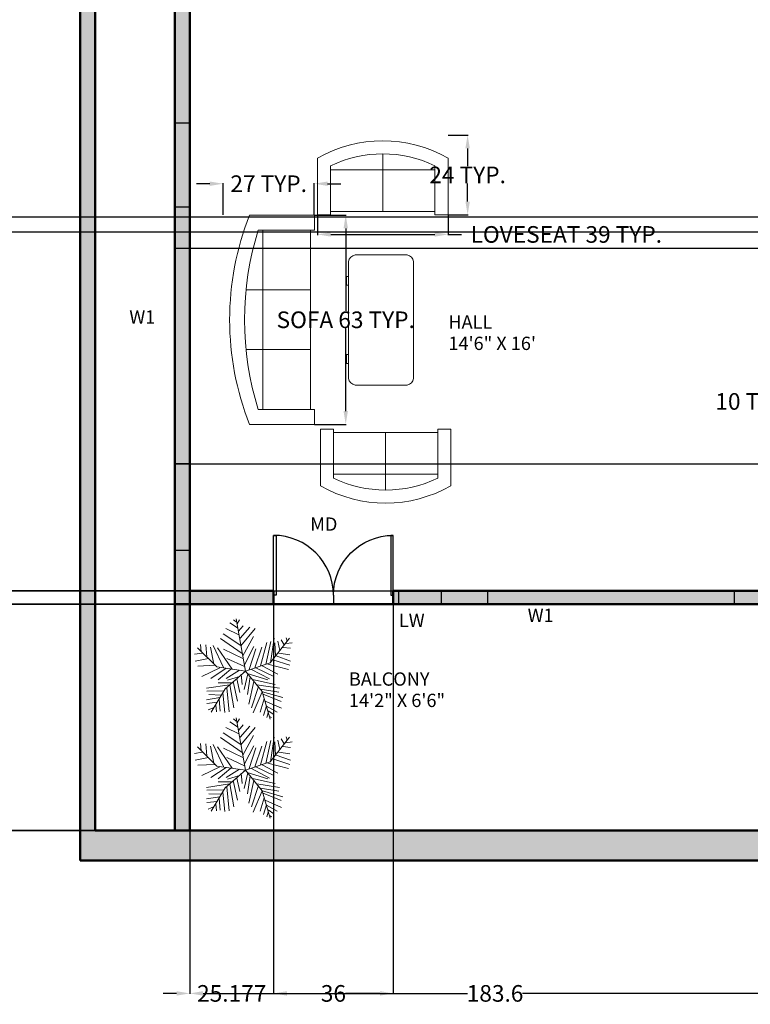
# Model space of a CAD drawing. Units: inches. Extents: x -12 to 887, y 330 to 874.
# Tile 5 of 9: x 442 to 662, y 330 to 626. Entities that reach past the tile are written whole.
import ezdxf

# ---------------------------------------------------------------- set-up
doc = ezdxf.new("R2010")
doc.units = ezdxf.units.IN
doc.header["$MEASUREMENT"] = 0
for name, color, linetype, lineweight in [('A-ANNO-DIMS', 2, 'Continuous', 18), ('A-ANNO-TEXT', 3, 'Continuous', 18), ('A-AREA-IDEN', 7, 'Continuous', 18), ('A-DOOR', 4, 'Continuous', 25), ('A-FURN', 9, 'Continuous', 18), ('A-GLAZ', 4, 'Continuous', 25), ('A-WALL', 7, 'Continuous', 50), ('A-WALL-PATT', 5, 'Continuous', 13), ('L-PLNT', 3, 'Continuous', 13)]:
    doc.layers.add(name, color=color, linetype=linetype, lineweight=lineweight)
doc.styles.get("Standard").update_dxf_attribs({"font": 'arial.ttf'})
doc.dimstyles.get("Standard").update_dxf_attribs({"dimtxt": 5, "dimasz": 4, "dimexe": 0.18, "dimexo": 0.0625, "dimgap": 0.09, "dimtad": 0, "dimtih": 1, "dimtoh": 1, "dimdec": 1, "dimzin": 0, "dimdsep": 46, "dimlunit": 4, "dimtxsty": 'Standard', "dimcen": 0.09, "dimadec": 0, "dimazin": 0, "dimtfac": 1, "dimtdec": 1, "dimtofl": 0, "dimtmove": 0, "dimatfit": 3, "dimfxl": 1, "dimtolj": 1, "dimtzin": 0, "dimarcsym": 0})

# ---------------------------------------------------------------- blocks, each defined once
blk = doc.blocks.new('*U5')
for p, q in [((0, 0), (0, -6)), ((40, 0), (40, -6))]:
    blk.add_line(p, q)
blk.add_lwpolyline([(0, 0), (0, 40), (1.75, 40), (1.75, 0)], close=True)
blk.add_arc((0, 0), 40, 0, 90)
blk = doc.blocks.new('Sofa - Roundback 7 ft.')
for p, q in [((-12.00002, -32.4421), (-12.00003, -6.5971)), ((11.99997, -32.4421), (11.99998, -6.5971)), ((-36.000027, -34), (-36.000027, -11.4696)), ((35.99998, -34), (35.99998, -11.4696)), ((-35.999844, -13.3819), (35.9998, -13.3819)), ((-36.000027, -32.4421), (35.99998, -32.4421))]:
    blk.add_line(p, q)
for points in [[(-36.000027, -34), (-42.000027, -34), (-42.000027, -8)], [(41.99998, -8), (41.99998, -34), (35.99998, -34)]]:
    blk.add_lwpolyline(points)
for centre, radius, start, end in [((0, -114.25), 114.25, 68.43141, 111.5686), ((-0.00001, -127.1968), 121.1968, 72.72033, 107.2797)]:
    blk.add_arc(centre, radius, start, end)
blk = doc.blocks.new('Sofa - Roundback Loveseat 5 ft.')
for p, q in [((0, -32.44198), (0, -5.99998)), ((-24, -33.99998), (-24, -11.46958)), ((-23.9998, -13.38178), (23.99986, -13.38178)), ((24.00004, -33.99998), (24.00004, -11.46958)), ((-24, -32.44198), (24.00004, -32.44198))]:
    blk.add_line(p, q)
for points in [[(-24, -33.99998), (-30, -33.99998), (-30, -7.99998)], [(30.00004, -7.99998), (30.00004, -33.99998), (24.00004, -33.99998)]]:
    blk.add_lwpolyline(points)
for centre, radius, start, end in [((0, -60.24998), 60.24998, 60.13715, 119.8628), ((0, -61.38438), 55.38444, 64.32083, 115.6792)]:
    blk.add_arc(centre, radius, start, end)
blk = doc.blocks.new('Desk - 30 x 60 in.')
for p, q in [((-26.999995, 0), (26.999995, 0)), ((-29.999995, -27), (-29.999995, -3)), ((29.999995, -3), (29.999995, -27)), ((26.999995, -30), (-26.999995, -30)), ((-20.000005, -30), (-20.000005, -31)), ((-20.000005, -31), (-16.000005, -31)), ((-16.000005, -31), (-16.000005, -30)), ((15.999995, -31), (15.999995, -30)), ((19.999995, -31), (15.999995, -31)), ((19.999995, -30), (19.999995, -31))]:
    blk.add_line(p, q)
for centre, start, end in [((-26.499995, -3.5), 98.1301, 171.8699), ((26.499995, -3.5), 8.130102, 81.8699), ((-26.499995, -26.5), 188.1301, 261.8699), ((26.499995, -26.5), 278.1301, 351.8699)]:
    blk.add_arc(centre, 3.535534, start, end)
blk = doc.blocks.new('*U14')
for p, q in [((-258.7244, 1362.456), (-332.3336, 1421.4348)), ((0, 0), (-266.7, 1447.8)), ((-231.1146, 1315.2628), (-166.7002, 1421.4348)), ((-185.1152, 1008.5578), (-553.1612, 1185.4942)), ((-221.9198, 1197.3052), (-433.5526, 1338.8594)), ((-194.31, 1102.9442), (-65.4812, 1256.284)), ((-148.3106, 914.1968), (118.5418, 1220.9018)), ((-129.8956, 701.8528), (265.7602, 1185.4942)), ((-93.091, 489.5342), (-700.3796, 902.3858)), ((-129.8956, 713.6638), (-626.7704, 1032.1544)), ((-74.7014, 418.7444), (219.7608, 961.39)), ((560.197, 182.8292), (698.2206, 819.8358)), ((685.8, 228.6), (1219.2, 914.4)), ((689.0258, 230.0224), (790.2448, 914.1968)), ((891.4384, 831.6214), (946.658, 572.1096)), ((983.4626, 867.0036), (1066.2666, 725.4494)), ((1121.4862, 925.9824), (1149.0706, 831.6214)), ((-800.1, 114.3), (-1333.5, 647.7)), ((-1234.059, 536.7274), (-1252.4486, 737.2604)), ((-1105.2302, 725.4494), (-1077.6458, 395.1732)), ((-976.4268, 666.4706), (-884.4026, 194.6402)), ((-902.8176, 713.6638), (-617.5756, 100.2538)), ((-369.1382, 53.086), (-783.1836, 642.874)), ((-617.5756, 607.4918), (-74.7014, 347.98)), ((-28.6766, 171.0436), (228.9556, 678.2816)), ((100.1268, 41.275), (284.1498, 619.2774)), ((256.5654, 88.4682), (449.7832, 666.4706)), ((412.9786, 147.447), (587.8068, 796.2392)), ((808.6344, 784.4282), (827.0494, 418.7444)), ((1029.462, 654.685), (1241.0948, 631.0884)), ((1112.2914, 760.8316), (1296.3144, 784.4282)), ((-1206.4492, 501.3198), (-1418.082, 465.9376)), ((-1031.621, 347.98), (-1399.667, 277.1902)), ((-525.5514, 347.98), (-28.6766, 123.8504)), ((753.4148, 312.5978), (1222.6798, 159.2326)), ((845.439, 418.7444), (1241.0948, 277.1902)), ((919.0482, 501.3198), (1222.6798, 454.152)), ((-847.598, 159.2326), (-1326.0578, 135.636)), ((-718.7946, 88.4682), (-1215.644, -147.447)), ((-543.9664, 76.6572), (-967.2066, -206.4512)), ((0, 0), (-800.1, 114.3)), ((-405.9428, 53.086), (-764.794, -241.8334)), ((0, 0), (-571.5, -495.3)), ((-166.7002, 29.4894), (-543.9664, -206.4512)), ((0, 0), (685.8, 228.6)), ((0, 0), (457.2, -571.5)), ((164.5412, 41.275), (661.416, -218.2368)), ((284.1498, 88.4682), (781.0246, -147.447)), ((458.978, 147.447), (891.4384, -88.4682)), ((615.4166, 194.6402), (1185.8752, 41.275)), ((-166.7002, -147.447), (-507.1618, -253.619)), ((-240.3094, -218.2368), (-157.5054, -595.7062)), ((-120.7008, -88.4682), (-93.091, -371.5766)), ((63.3222, -76.6826), (-37.8714, -513.1308)), ((44.9326, -64.897), (615.4166, -241.8334)), ((127.7366, -159.258), (54.1274, -654.685)), ((192.151, -230.0224), (817.8292, -371.5766)), ((-442.7474, -383.3876), (-1086.8406, -477.7486)), ((-571.5, -495.3), (-952.5, -1143)), ((-387.5278, -324.4088), (-764.794, -324.4088)), ((-525.5514, -465.963), (-451.9422, -1126.5408)), ((-433.5526, -383.3876), (-323.1134, -1020.3688)), ((-341.5284, -289.0012), (-221.9198, -831.6214)), ((228.9556, -289.0012), (90.932, -914.1968)), ((357.759, -430.5554), (164.5412, -1020.3688)), ((311.7596, -383.3876), (937.4378, -477.7486)), ((412.9786, -501.3452), (919.0482, -583.9206)), ((-718.7946, -737.2604), (-1086.8406, -796.2392)), ((-617.5756, -548.5384), (-1077.6458, -560.324)), ((-681.9646, -666.496), (-1022.4262, -654.685)), ((-737.1842, -784.4536), (-709.5744, -1114.7298)), ((-635.9652, -607.5172), (-580.771, -1150.1374)), ((458.978, -572.1096), (210.5406, -1161.923)), ((514.1976, -772.6426), (403.7838, -1138.3264)), ((457.2, -571.5), (685.8, -1333.5)), ((468.1982, -572.1096), (1029.462, -737.2604)), ((486.5878, -642.8994), (983.4626, -843.4324)), ((-783.1836, -867.029), (-1077.6458, -902.4112)), ((-875.2078, -1008.5832), (-1040.8412, -1079.3476)), ((-829.2084, -937.7934), (-810.7934, -1126.5408)), ((578.612, -961.39), (495.7826, -1232.7128)), ((541.8074, -831.6214), (992.6574, -1032.1544)), ((578.612, -973.1756), (873.0488, -1138.3264)), ((624.6114, -1161.923), (587.8068, -1291.6916)), ((624.6114, -1102.9442), (781.0246, -1209.1162)), ((679.8056, -1268.095), (716.6102, -1291.6916))]:
    blk.add_line(p, q)
blk = doc.blocks.new('*D19')
at = {"layer": 'A-ANNO-DIMS', "color": 0, "lineweight": -2, "transparency": 16777216}
for p, q in [((678.65, 512.63), (678.65, 510.96)), ((688.99, 512.63), (688.99, 510.96)), ((678.65, 511.14), (674.65, 511.14)), ((684.99, 511.14), (682.65, 511.14))]:
    blk.add_line(p, q, dxfattribs=at)
at = {"layer": 'A-ANNO-DIMS', "color": 0, "transparency": 16777216}
for points in [[(682.65, 511.8), (682.65, 510.47), (678.65, 511.14)], [(684.99, 511.8), (684.99, 510.47), (688.99, 511.14)]]:
    blk.add_solid(points, dxfattribs=at)
at = {"layer": 'Defpoints', "color": 0, "transparency": 16777216}
for p in [(678.65, 512.69), (688.99, 512.69), (678.65, 511.14)]:
    blk.add_point(p, dxfattribs=at)
at = {"layer": 'A-ANNO-DIMS', "color": 0, "transparency": 16777216, "insert": (662.62, 511.14), "char_height": 5, "attachment_point": 5}
blk.add_mtext('\\A1;10 TYP.', dxfattribs=at)
blk = doc.blocks.new('*D30')
at = {"layer": 'A-ANNO-DIMS', "color": 0, "lineweight": -2, "transparency": 16777216}
for p, q in [((530.58, 567.16), (540.13, 567.16)), ((539.95, 563.16), (539.95, 538.37)), ((539.95, 508.23), (539.95, 533.02)), ((530.58, 504.23), (540.13, 504.23))]:
    blk.add_line(p, q, dxfattribs=at)
at = {"layer": 'A-ANNO-DIMS', "color": 0, "transparency": 16777216}
for points in [[(539.29, 563.16), (540.62, 563.16), (539.95, 567.16)], [(539.29, 508.23), (540.62, 508.23), (539.95, 504.23)]]:
    blk.add_solid(points, dxfattribs=at)
at = {"layer": 'Defpoints', "color": 0, "transparency": 16777216}
for p in [(530.51, 567.16), (539.95, 567.16), (530.51, 504.23)]:
    blk.add_point(p, dxfattribs=at)
at = {"layer": 'A-ANNO-DIMS', "color": 0, "transparency": 16777216, "insert": (539.95, 535.69), "char_height": 5, "attachment_point": 5}
blk.add_mtext('\\A1;SOFA 63 TYP.', dxfattribs=at)
blk = doc.blocks.new('*D31')
at = {"layer": 'A-ANNO-DIMS', "color": 0, "lineweight": -2, "transparency": 16777216}
for p, q in [((499.05, 576.6), (495.05, 576.6)), ((503.05, 567.22), (503.05, 576.78)), ((530.51, 567.22), (530.51, 576.78)), ((534.51, 576.6), (538.51, 576.6))]:
    blk.add_line(p, q, dxfattribs=at)
at = {"layer": 'A-ANNO-DIMS', "color": 0, "transparency": 16777216}
for points in [[(499.05, 577.26), (499.05, 575.93), (503.05, 576.6)], [(534.51, 577.26), (534.51, 575.93), (530.51, 576.6)]]:
    blk.add_solid(points, dxfattribs=at)
at = {"layer": 'Defpoints', "color": 0, "transparency": 16777216}
for p in [(503.05, 576.6), (503.05, 567.16), (530.51, 567.16)]:
    blk.add_point(p, dxfattribs=at)
at = {"layer": 'A-ANNO-DIMS', "color": 0, "transparency": 16777216, "insert": (516.78, 576.6), "char_height": 5, "attachment_point": 5}
blk.add_mtext('\\A1;27 TYP.', dxfattribs=at)
blk = doc.blocks.new('*D32')
at = {"layer": 'A-ANNO-DIMS', "color": 0, "lineweight": -2, "transparency": 16777216}
for p, q in [((531.45, 567.18), (531.45, 561.17)), ((570.72, 567.18), (570.72, 561.17)), ((535.45, 561.35), (566.72, 561.35)), ((570.72, 561.35), (574.72, 561.35))]:
    blk.add_line(p, q, dxfattribs=at)
at = {"layer": 'A-ANNO-DIMS', "color": 0, "transparency": 16777216}
for points in [[(535.45, 562.02), (535.45, 560.68), (531.45, 561.35)], [(566.72, 562.02), (566.72, 560.68), (570.72, 561.35)]]:
    blk.add_solid(points, dxfattribs=at)
at = {"layer": 'Defpoints', "color": 0, "transparency": 16777216}
for p in [(531.45, 567.24), (570.72, 567.24), (570.72, 561.35)]:
    blk.add_point(p, dxfattribs=at)
at = {"layer": 'A-ANNO-DIMS', "color": 0, "transparency": 16777216, "insert": (606.28, 561.35), "char_height": 5, "attachment_point": 5}
blk.add_mtext('\\A1;LOVESEAT 39 TYP.', dxfattribs=at)
blk = doc.blocks.new('*D33')
at = {"layer": 'A-ANNO-DIMS', "color": 0, "lineweight": -2, "transparency": 16777216}
for p, q in [((570.78, 591.23), (576.79, 591.23)), ((576.61, 587.23), (576.61, 581.84)), ((576.61, 571.24), (576.61, 576.63)), ((570.78, 567.24), (576.79, 567.24))]:
    blk.add_line(p, q, dxfattribs=at)
at = {"layer": 'A-ANNO-DIMS', "color": 0, "transparency": 16777216}
for points in [[(575.94, 587.23), (577.28, 587.23), (576.61, 591.23)], [(575.94, 571.24), (577.28, 571.24), (576.61, 567.24)]]:
    blk.add_solid(points, dxfattribs=at)
at = {"layer": 'Defpoints', "color": 0, "transparency": 16777216}
for p in [(570.72, 591.23), (576.61, 591.23), (570.72, 567.24)]:
    blk.add_point(p, dxfattribs=at)
at = {"layer": 'A-ANNO-DIMS', "color": 0, "transparency": 16777216, "insert": (576.61, 579.24), "char_height": 5, "attachment_point": 5}
blk.add_mtext('\\A1;24 TYP.', dxfattribs=at)
blk = doc.blocks.new('*D60')
at = {"layer": 'A-ANNO-DIMS', "color": 0, "lineweight": -2, "transparency": 16777216}
for p, q in [((383.99, 450.16), (873.75, 450.16)), ((873.57, 446.16), (873.57, 418.8)), ((873.57, 386.16), (873.57, 413.52)), ((383.99, 382.16), (873.75, 382.16))]:
    blk.add_line(p, q, dxfattribs=at)
at = {"layer": 'A-ANNO-DIMS', "color": 0, "transparency": 16777216}
for points in [[(872.9, 446.16), (874.24, 446.16), (873.57, 450.16)], [(872.9, 386.16), (874.24, 386.16), (873.57, 382.16)]]:
    blk.add_solid(points, dxfattribs=at)
at = {"layer": 'Defpoints', "color": 0, "transparency": 16777216}
for p in [(383.93, 450.16), (873.57, 450.16), (383.93, 382.16)]:
    blk.add_point(p, dxfattribs=at)
at = {"layer": 'A-ANNO-DIMS', "color": 0, "transparency": 16777216, "insert": (873.57, 416.16), "char_height": 5, "attachment_point": 5}
blk.add_mtext('\\A1;68', dxfattribs=at)
blk = doc.blocks.new('*D61')
at = {"layer": 'A-ANNO-DIMS', "color": 0, "lineweight": -2, "transparency": 16777216}
for p, q in [((873.57, 458.16), (873.57, 462.16)), ((873.57, 462.16), (877.57, 462.16)), ((383.99, 454.16), (873.75, 454.16)), ((383.99, 450.16), (873.75, 450.16)), ((873.57, 446.16), (873.57, 442.16))]:
    blk.add_line(p, q, dxfattribs=at)
at = {"layer": 'A-ANNO-DIMS', "color": 0, "transparency": 16777216}
for points in [[(872.9, 458.16), (874.24, 458.16), (873.57, 454.16)], [(872.9, 446.16), (874.24, 446.16), (873.57, 450.16)]]:
    blk.add_solid(points, dxfattribs=at)
at = {"layer": 'Defpoints', "color": 0, "transparency": 16777216}
for p in [(383.93, 454.16), (873.57, 454.16), (383.93, 450.16)]:
    blk.add_point(p, dxfattribs=at)
at = {"layer": 'A-ANNO-DIMS', "color": 0, "transparency": 16777216, "insert": (879.39, 462.16), "char_height": 5, "attachment_point": 5}
blk.add_mtext('\\A1;4', dxfattribs=at)
blk = doc.blocks.new('*D62')
at = {"layer": 'A-ANNO-DIMS', "color": 0, "lineweight": -2, "transparency": 16777216}
for p, q in [((383.99, 562.16), (873.75, 562.16)), ((873.57, 558.16), (873.57, 510.8)), ((873.57, 458.16), (873.57, 505.52)), ((383.99, 454.16), (873.75, 454.16))]:
    blk.add_line(p, q, dxfattribs=at)
at = {"layer": 'A-ANNO-DIMS', "color": 0, "transparency": 16777216}
for points in [[(872.9, 558.16), (874.24, 558.16), (873.57, 562.16)], [(872.9, 458.16), (874.24, 458.16), (873.57, 454.16)]]:
    blk.add_solid(points, dxfattribs=at)
at = {"layer": 'Defpoints', "color": 0, "transparency": 16777216}
for p in [(383.93, 562.16), (873.57, 562.16), (383.93, 454.16)]:
    blk.add_point(p, dxfattribs=at)
at = {"layer": 'A-ANNO-DIMS', "color": 0, "transparency": 16777216, "insert": (873.57, 508.16), "char_height": 5, "attachment_point": 5}
blk.add_mtext('\\A1;108', dxfattribs=at)
blk = doc.blocks.new('*D63')
at = {"layer": 'A-ANNO-DIMS', "color": 0, "lineweight": -2, "transparency": 16777216}
for p, q in [((873.57, 570.66), (873.57, 574.66)), ((873.57, 574.66), (877.57, 574.66)), ((383.99, 566.66), (873.75, 566.66)), ((383.99, 562.16), (873.75, 562.16)), ((873.57, 558.16), (873.57, 554.16))]:
    blk.add_line(p, q, dxfattribs=at)
at = {"layer": 'A-ANNO-DIMS', "color": 0, "transparency": 16777216}
for points in [[(872.9, 570.66), (874.24, 570.66), (873.57, 566.66)], [(872.9, 558.16), (874.24, 558.16), (873.57, 562.16)]]:
    blk.add_solid(points, dxfattribs=at)
at = {"layer": 'Defpoints', "color": 0, "transparency": 16777216}
for p in [(383.93, 566.66), (873.57, 566.66), (383.93, 562.16)]:
    blk.add_point(p, dxfattribs=at)
at = {"layer": 'A-ANNO-DIMS', "color": 0, "transparency": 16777216, "insert": (882.33, 574.66), "char_height": 5, "attachment_point": 5}
blk.add_mtext('\\A1;4.5', dxfattribs=at)
blk = doc.blocks.new('*D64')
at = {"layer": 'A-ANNO-DIMS', "color": 0, "lineweight": -2, "transparency": 16777216}
for p, q in [((383.99, 685.16), (873.75, 685.16)), ((873.57, 681.16), (873.57, 628.55)), ((873.57, 570.66), (873.57, 623.27)), ((383.99, 566.66), (873.75, 566.66))]:
    blk.add_line(p, q, dxfattribs=at)
at = {"layer": 'A-ANNO-DIMS', "color": 0, "transparency": 16777216}
for points in [[(872.9, 681.16), (874.24, 681.16), (873.57, 685.16)], [(872.9, 570.66), (874.24, 570.66), (873.57, 566.66)]]:
    blk.add_solid(points, dxfattribs=at)
at = {"layer": 'Defpoints', "color": 0, "transparency": 16777216}
for p in [(383.93, 685.16), (873.57, 685.16), (383.93, 566.66)]:
    blk.add_point(p, dxfattribs=at)
at = {"layer": 'A-ANNO-DIMS', "color": 0, "transparency": 16777216, "insert": (873.57, 625.91), "char_height": 5, "attachment_point": 5}
blk.add_mtext('\\A1;118.5', dxfattribs=at)
blk = doc.blocks.new('*D95')
at = {"layer": 'A-ANNO-DIMS', "color": 0, "lineweight": -2, "transparency": 16777216}
for p, q in [((493.07, 382.1), (493.07, 332.98)), ((676.66, 382.1), (676.66, 332.98)), ((497.07, 333.16), (576.57, 333.16)), ((672.66, 333.16), (593.15, 333.16))]:
    blk.add_line(p, q, dxfattribs=at)
at = {"layer": 'A-ANNO-DIMS', "color": 0, "transparency": 16777216}
for points in [[(497.07, 333.83), (497.07, 332.49), (493.07, 333.16)], [(672.66, 333.83), (672.66, 332.49), (676.66, 333.16)]]:
    blk.add_solid(points, dxfattribs=at)
at = {"layer": 'Defpoints', "color": 0, "transparency": 16777216}
for p in [(493.07, 382.16), (676.66, 382.16), (676.66, 333.16)]:
    blk.add_point(p, dxfattribs=at)
at = {"layer": 'A-ANNO-DIMS', "color": 0, "transparency": 16777216, "insert": (584.86, 333.16), "char_height": 5, "attachment_point": 5}
blk.add_mtext('\\A1;183.6', dxfattribs=at)
blk = doc.blocks.new('*D98')
at = {"layer": 'A-ANNO-DIMS', "color": 0, "lineweight": -2, "transparency": 16777216}
for p, q in [((460.13, 830.66), (873.75, 830.66)), ((873.57, 826.66), (873.57, 604.54)), ((873.57, 377.16), (873.57, 599.28)), ((460.13, 373.16), (873.75, 373.16))]:
    blk.add_line(p, q, dxfattribs=at)
at = {"layer": 'A-ANNO-DIMS', "color": 0, "transparency": 16777216}
for points in [[(872.9, 826.66), (874.24, 826.66), (873.57, 830.66)], [(872.9, 377.16), (874.24, 377.16), (873.57, 373.16)]]:
    blk.add_solid(points, dxfattribs=at)
at = {"layer": 'Defpoints', "color": 0, "transparency": 16777216}
for p in [(460.07, 830.66), (873.57, 830.66), (460.07, 373.16)]:
    blk.add_point(p, dxfattribs=at)
at = {"layer": 'A-ANNO-DIMS', "color": 0, "transparency": 16777216, "insert": (873.57, 601.91), "char_height": 5, "attachment_point": 5}
blk.add_mtext('\\A1;457.5', dxfattribs=at)
blk = doc.blocks.new('*D99')
at = {"layer": 'A-ANNO-DIMS', "color": 0, "lineweight": -2, "transparency": 16777216}
for p, q in [((493.01, 450.16), (1.75, 450.16)), ((1.93, 446.16), (1.93, 418.8)), ((1.93, 386.16), (1.93, 413.52)), ((493.01, 382.16), (1.75, 382.16))]:
    blk.add_line(p, q, dxfattribs=at)
at = {"layer": 'A-ANNO-DIMS', "color": 0, "transparency": 16777216}
for points in [[(1.26, 446.16), (2.59, 446.16), (1.93, 450.16)], [(1.26, 386.16), (2.59, 386.16), (1.93, 382.16)]]:
    blk.add_solid(points, dxfattribs=at)
at = {"layer": 'Defpoints', "color": 0, "transparency": 16777216}
for p in [(1.93, 450.16), (493.07, 450.16), (493.07, 382.16)]:
    blk.add_point(p, dxfattribs=at)
at = {"layer": 'A-ANNO-DIMS', "color": 0, "transparency": 16777216, "insert": (1.93, 416.16), "char_height": 5, "attachment_point": 5}
blk.add_mtext('\\A1;68', dxfattribs=at)
blk = doc.blocks.new('*D100')
at = {"layer": 'A-ANNO-DIMS', "color": 0, "lineweight": -2, "transparency": 16777216}
for p, q in [((1.93, 458.16), (1.93, 462.16)), ((1.93, 462.16), (5.93, 462.16)), ((493.01, 454.16), (1.75, 454.16)), ((493.01, 450.16), (1.75, 450.16)), ((1.93, 446.16), (1.93, 442.16))]:
    blk.add_line(p, q, dxfattribs=at)
at = {"layer": 'A-ANNO-DIMS', "color": 0, "transparency": 16777216}
for points in [[(1.26, 458.16), (2.59, 458.16), (1.93, 454.16)], [(1.26, 446.16), (2.59, 446.16), (1.93, 450.16)]]:
    blk.add_solid(points, dxfattribs=at)
at = {"layer": 'Defpoints', "color": 0, "transparency": 16777216}
for p in [(1.93, 454.16), (493.07, 454.16), (493.07, 450.16)]:
    blk.add_point(p, dxfattribs=at)
at = {"layer": 'A-ANNO-DIMS', "color": 0, "transparency": 16777216, "insert": (7.75, 462.16), "char_height": 5, "attachment_point": 5}
blk.add_mtext('\\A1;4', dxfattribs=at)
blk = doc.blocks.new('*D101')
at = {"layer": 'A-ANNO-DIMS', "color": 0, "lineweight": -2, "transparency": 16777216}
for p, q in [((493.01, 643.16), (1.75, 643.16)), ((1.93, 639.16), (1.93, 551.3)), ((1.93, 458.16), (1.93, 546.02)), ((493.01, 454.16), (1.75, 454.16))]:
    blk.add_line(p, q, dxfattribs=at)
at = {"layer": 'A-ANNO-DIMS', "color": 0, "transparency": 16777216}
for points in [[(1.26, 639.16), (2.59, 639.16), (1.93, 643.16)], [(1.26, 458.16), (2.59, 458.16), (1.93, 454.16)]]:
    blk.add_solid(points, dxfattribs=at)
at = {"layer": 'Defpoints', "color": 0, "transparency": 16777216}
for p in [(1.93, 643.16), (493.07, 643.16), (493.07, 454.16)]:
    blk.add_point(p, dxfattribs=at)
at = {"layer": 'A-ANNO-DIMS', "color": 0, "transparency": 16777216, "insert": (1.93, 548.66), "char_height": 5, "attachment_point": 5}
blk.add_mtext('\\A1;189', dxfattribs=at)
blk = doc.blocks.new('*D120')
at = {"layer": 'A-ANNO-DIMS', "color": 0, "lineweight": -2, "transparency": 16777216}
for p, q in [((518.25, 454.1), (518.25, 332.98)), ((554.25, 454.1), (554.25, 332.98)), ((522.25, 333.16), (532.58, 333.16)), ((550.25, 333.16), (539.91, 333.16))]:
    blk.add_line(p, q, dxfattribs=at)
at = {"layer": 'A-ANNO-DIMS', "color": 0, "transparency": 16777216}
for points in [[(522.25, 333.83), (522.25, 332.49), (518.25, 333.16)], [(550.25, 333.83), (550.25, 332.49), (554.25, 333.16)]]:
    blk.add_solid(points, dxfattribs=at)
at = {"layer": 'Defpoints', "color": 0, "transparency": 16777216}
for p in [(518.25, 454.16), (554.25, 454.16), (554.25, 333.16)]:
    blk.add_point(p, dxfattribs=at)
at = {"layer": 'A-ANNO-DIMS', "color": 0, "transparency": 16777216, "insert": (536.25, 333.16), "char_height": 5, "attachment_point": 5}
blk.add_mtext('\\A1;36', dxfattribs=at)
blk = doc.blocks.new('*D121')
at = {"layer": 'A-ANNO-DIMS', "color": 0, "lineweight": -2, "transparency": 16777216}
for p, q in [((493.07, 454.1), (493.07, 332.98)), ((518.25, 454.1), (518.25, 332.98)), ((489.07, 333.16), (485.07, 333.16)), ((522.25, 333.16), (526.25, 333.16))]:
    blk.add_line(p, q, dxfattribs=at)
at = {"layer": 'A-ANNO-DIMS', "color": 0, "transparency": 16777216}
for points in [[(489.07, 333.83), (489.07, 332.49), (493.07, 333.16)], [(522.25, 333.83), (522.25, 332.49), (518.25, 333.16)]]:
    blk.add_solid(points, dxfattribs=at)
at = {"layer": 'Defpoints', "color": 0, "transparency": 16777216}
for p in [(493.07, 454.16), (518.25, 454.16), (518.25, 333.16)]:
    blk.add_point(p, dxfattribs=at)
at = {"layer": 'A-ANNO-DIMS', "color": 0, "transparency": 16777216, "insert": (505.66, 333.16), "char_height": 5, "attachment_point": 5}
blk.add_mtext('\\A1;25.177', dxfattribs=at)
blk = doc.blocks.new('*D129')
at = {"layer": 'A-ANNO-DIMS', "color": 0, "lineweight": -2, "transparency": 16777216}
for p, q in [((488.63, 557.26), (873.75, 557.26)), ((873.57, 553.26), (873.57, 527.44)), ((873.57, 496.34), (873.57, 522.16)), ((488.63, 492.34), (873.75, 492.34))]:
    blk.add_line(p, q, dxfattribs=at)
at = {"layer": 'A-ANNO-DIMS', "color": 0, "transparency": 16777216}
for points in [[(872.9, 553.26), (874.24, 553.26), (873.57, 557.26)], [(872.9, 496.34), (874.24, 496.34), (873.57, 492.34)]]:
    blk.add_solid(points, dxfattribs=at)
at = {"layer": 'Defpoints', "color": 0, "transparency": 16777216}
for p in [(488.57, 557.26), (488.57, 492.34), (873.57, 492.34)]:
    blk.add_point(p, dxfattribs=at)
at = {"layer": 'A-ANNO-DIMS', "color": 0, "transparency": 16777216, "insert": (873.57, 524.8), "char_height": 5, "attachment_point": 5}
blk.add_mtext('\\A1;64.91', dxfattribs=at)

msp = doc.modelspace()

# ---------------------------------------------------------------- hatches: boundary and pattern name
at = {"layer": 'A-WALL-PATT'}
h = msp.add_hatch(color=256, dxfattribs=at)
h.dxf.hatch_style = 1
h.paths.add_polyline_path([(94.575, 830.6611), (67.3199, 830.6611), (67.3199, 821.6611), (70.4263, 821.6611), (79.4263, 821.6611), (94.575, 821.6611)])
h.paths.add_polyline_path([(288.8031, 830.6611), (257.9263, 830.6611), (253.4263, 830.6611), (253.4263, 821.6611), (288.8031, 821.6611)])
h.paths.add_polyline_path([(74.9263, 696.9265), (70.4263, 696.9265), (70.4263, 678.4656), (74.9263, 678.4656)])
h.paths.add_polyline_path([(74.9263, 584.8756), (70.4263, 584.8756), (70.4263, 562.1611), (74.9263, 562.1611)])
h.paths.add_polyline_path([(135.5357, 566.6611), (122.6994, 566.6611), (122.6994, 562.1611), (135.5357, 562.1611)])
h.paths.add_polyline_path([(257.9263, 579.1607), (253.4263, 579.1607), (253.4263, 562.1611), (257.9263, 562.1611)])
h.paths.add_polyline_path([(272.0195, 454.1611), (254.2006, 454.1611), (254.2006, 450.1611), (272.0195, 450.1611)])
h.paths.add_polyline_path([(392.9263, 454.1611), (374.959, 454.1611), (374.959, 450.1611), (383.9263, 450.1611), (392.9263, 450.1611)])
h.paths.add_polyline_path([(493.0683, 466.4171), (488.5683, 466.4171), (488.5683, 450.1611), (493.0683, 450.1611)])
h.paths.add_polyline_path([(568.6302, 454.1611), (555.938, 454.1611), (555.938, 450.1611), (568.6302, 450.1611)])
h.paths.add_polyline_path([(493.0683, 594.9471), (488.5683, 594.9471), (488.5683, 569.5862), (493.0683, 569.5862)])
h.paths.add_polyline_path([(690.1615, 454.1611), (672.3426, 454.1611), (672.3426, 450.1611), (690.1615, 450.1611)])
h.paths.add_polyline_path([(811.0683, 454.1611), (793.101, 454.1611), (793.101, 450.1611), (802.0683, 450.1611), (811.0683, 450.1611)])
h.paths.add_polyline_path([(811.0683, 578.3606), (802.0683, 578.3606), (802.0683, 566.6611), (802.0683, 553.5254), (811.0683, 553.5254)])
h.paths.add_polyline_path([(811.0683, 701.6611), (802.0683, 701.6611), (802.0683, 689.9616), (802.0683, 676.8259), (811.0683, 676.8259)])
h.paths.add_polyline_path([(811.0683, 830.6611), (782.165, 830.6611), (782.165, 821.6611), (802.0683, 821.6611), (811.0683, 821.6611)])
h.paths.add_polyline_path([(706.9451, 830.6611), (671.5683, 830.6611), (671.5683, 821.6611), (706.9451, 821.6611)])
h.paths.add_polyline_path([(512.717, 830.6611), (485.4619, 830.6611), (485.4619, 821.6611), (488.5683, 821.6611), (512.717, 821.6611)])
h.paths.add_polyline_path([(392.9263, 697.8668), (383.9263, 697.8668), (383.9263, 689.6611), (383.9263, 676.5034), (392.9263, 676.5034)])
h.paths.add_polyline_path([(392.9263, 830.6611), (364.023, 830.6611), (364.023, 821.7357), (392.9263, 821.7357)])
h.paths.add_polyline_path([(392.9263, 619.0434), (383.9263, 619.0434), (383.9263, 588.7499), (392.9263, 588.7499)])
h.paths.add_polyline_path([(392.9263, 578.3606), (383.9263, 578.3606), (383.9263, 566.6611), (383.9263, 553.5254), (392.9263, 553.5254)])
h.paths.add_polyline_path([(257.9263, 699.8547), (253.4263, 699.8547), (253.4263, 697.1611), (253.4263, 677.338), (257.9263, 677.338)])
h.paths.add_polyline_path([(493.0683, 714.3785), (488.5683, 714.3785), (488.5683, 689.6611), (493.0683, 689.6611)])
h.paths.add_polyline_path([(74.9263, 491.4191), (70.4263, 491.4191), (70.4263, 480.7097), (74.9263, 480.7097)])
h = msp.add_hatch(color=256, dxfattribs=at)
h.dxf.hatch_style = 1
h.paths.add_polyline_path([(671.5683, 830.6611), (512.717, 830.6611), (512.717, 821.6611), (617.0825, 821.6611), (617.0825, 797.5825), (617.0787, 783.3094), (621.5683, 783.3094), (621.5683, 821.6611), (671.5683, 821.6611)], flags=17)
h.paths.add_polyline_path([(833.5683, 830.6611), (811.0683, 830.6611), (811.0683, 821.6611), (829.0683, 821.6611), (829.0683, 701.6611), (829.0683, 382.1611), (811.0683, 382.1611), (811.0683, 450.1611), (802.0683, 450.1611), (802.0683, 382.1611), (671.5683, 382.1611), (464.5683, 382.1611), (464.5683, 821.6611), (460.0683, 821.6611), (460.0683, 373.1611), (671.5683, 373.1611), (833.5683, 373.1611)])
h.paths.add_polyline_path([(493.0683, 728.8273), (488.5683, 728.8273), (488.5683, 714.3785), (493.0683, 714.3785)], flags=17)
h.paths.add_polyline_path([(493.0683, 821.6611), (488.5683, 821.6611), (488.5683, 781.3634), (493.0683, 781.3634)], flags=17)
h = msp.add_hatch(color=256, dxfattribs=at)
h.dxf.hatch_style = 1
h.paths.add_polyline_path([(485.4619, 830.6611), (460.0683, 830.6611), (460.0683, 373.1611), (833.5683, 373.1611), (833.5683, 830.6611), (811.0683, 830.6611), (811.0683, 821.6611), (829.0683, 821.6611), (829.0683, 701.6611), (829.0683, 382.1611), (811.0683, 382.1611), (811.0683, 450.1611), (802.0683, 450.1611), (802.0683, 382.1611), (671.5683, 382.1611), (464.5683, 382.1611), (464.5683, 821.6611), (485.4619, 821.6611)])
h = msp.add_hatch(color=256, dxfattribs=at)
h.dxf.hatch_style = 1
h.paths.add_polyline_path([(671.5683, 749.6611), (621.5683, 749.6611), (621.5683, 759.3094), (620.6653, 759.3094), (617.0683, 759.3094), (617.0683, 745.1611), (671.5683, 745.1611)])
h.paths.add_polyline_path([(676.0683, 821.6611), (671.5683, 821.6611), (671.5683, 736.2424), (676.0683, 736.2424)])
h.paths.add_polyline_path([(782.165, 830.6611), (706.9451, 830.6611), (706.9451, 821.6611), (782.165, 821.6611)])
h.paths.add_polyline_path([(811.0683, 553.5254), (802.0683, 553.5254), (802.0683, 507.4529), (802.0683, 454.1611), (811.0683, 454.1611)])
h.paths.add_polyline_path([(793.101, 454.1611), (690.1615, 454.1611), (690.1615, 450.1611), (793.101, 450.1611)])
h.paths.add_polyline_path([(672.3426, 454.1611), (656.7304, 454.1611), (656.7304, 450.1611), (672.3426, 450.1611)])
h.paths.add_polyline_path([(582.6585, 454.1611), (568.6302, 454.1611), (568.6302, 450.1611), (582.6585, 450.1611)])
h.paths.add_polyline_path([(555.938, 454.1611), (554.2565, 454.1611), (554.2565, 452.8628), (554.2565, 450.1611), (555.938, 450.1611)])
h.paths.add_polyline_path([(518.2335, 452.8628), (518.2335, 454.1611), (493.0683, 454.1611), (493.0683, 450.1611), (518.2335, 450.1611)])
h.paths.add_polyline_path([(493.0683, 450.1611), (488.5683, 450.1611), (488.5683, 382.1611), (493.0683, 382.1611)])
h.paths.add_polyline_path([(493.0683, 492.3446), (488.5683, 492.3446), (488.5683, 466.4171), (493.0683, 466.4171)])
h.paths.add_polyline_path([(493.0683, 569.5862), (488.5683, 569.5862), (488.5683, 557.2595), (493.0683, 557.2595)])
h.paths.add_polyline_path([(493.0683, 689.6611), (488.5683, 689.6611), (488.5683, 594.9471), (493.0683, 594.9471)])
h.paths.add_polyline_path([(676.0683, 700.2227), (671.5683, 700.2227), (671.5683, 669.5589), (676.0683, 669.5589)])
h.paths.add_polyline_path([(739.0683, 689.6611), (676.0683, 689.6611), (676.0683, 685.1611), (739.0683, 685.1611)])
h.paths.add_polyline_path([(802.0683, 689.6611), (763.0683, 689.6611), (763.0683, 686.0698), (763.0683, 685.1611), (802.0683, 685.1611)])
h.paths.add_polyline_path([(811.0683, 821.6611), (802.0683, 821.6611), (802.0683, 756.0738), (811.0683, 756.0738)])
h.paths.add_polyline_path([(811.0683, 707.8935), (802.0683, 707.8935), (802.0683, 701.6611), (811.0683, 701.6611)])
h.paths.add_polyline_path([(811.0683, 676.8259), (802.0683, 676.8259), (802.0683, 628.1611), (730.0683, 628.1611), (730.0683, 623.6611), (802.0683, 623.6611), (802.0683, 578.3606), (811.0683, 578.3606)])
h.paths.add_polyline_path([(730.0683, 685.1611), (726.0683, 685.1611), (726.0683, 628.1611), (730.0683, 628.1611)])
h.paths.add_polyline_path([(724.0683, 685.1611), (720.0683, 685.1611), (720.0683, 628.1611), (724.0683, 628.1611)])
h.paths.add_polyline_path([(726.0683, 628.1611), (676.0683, 628.1611), (676.0683, 633.7662), (674.2492, 633.7662), (671.5683, 633.7662), (671.5683, 623.6611), (726.0683, 623.6611)])
h.paths.add_polyline_path([(730.0683, 628.1611), (726.0683, 628.1611), (726.0683, 623.6611), (730.0683, 623.6611)])
h.paths.add_polyline_path([(730.0683, 623.6611), (726.0683, 623.6611), (726.0683, 595.3822), (729.6731, 595.3822, -0.00411226), (730.0683, 595.379)])
h.paths.add_polyline_path([(802.0683, 564.6611), (730.0683, 564.6611), (730.0683, 571.3507), (729.6731, 571.3507), (726.0683, 571.3507), (726.0683, 564.6611), (718.522, 564.6611), (718.522, 560.1611), (802.0683, 560.1611)])
h.paths.add_polyline_path([(676.0683, 580.4772), (671.5683, 580.4772), (671.5683, 560.1611), (676.0683, 560.1611)])
h.paths.add_polyline_path([(682.5176, 564.6611), (676.0683, 564.6611), (676.0683, 560.1611), (682.5176, 560.1611)])
h.paths.add_polyline_path([(676.0683, 560.1611), (671.5683, 560.1611), (671.5683, 454.1611), (672.3426, 454.1611), (676.0683, 454.1611)])
h = msp.add_hatch(color=256, dxfattribs=at)
h.dxf.hatch_style = 1
h.paths.add_polyline_path([(74.9263, 749.8953), (70.4263, 749.8953), (70.4263, 709.2627), (74.9263, 709.2627)])
h.paths.add_polyline_path([(74.9263, 671.2153), (70.4263, 671.2153), (70.4263, 599.271), (74.9263, 599.271)])
h.paths.add_polyline_path([(229.0035, 566.6611), (142.5107, 566.6611), (142.5107, 562.1611), (229.0035, 562.1611)])
h.paths.add_polyline_path([(392.9263, 742.7561), (383.9263, 742.7561), (383.9263, 706.6608), (392.9263, 706.6608)])
h.paths.add_polyline_path([(656.7304, 454.1611), (582.6585, 454.1611), (582.6585, 450.1611), (656.7304, 450.1611)])
h.paths.add_polyline_path([(493.0683, 557.2595), (488.5683, 557.2595), (488.5683, 492.3446), (493.0683, 492.3446)])
h.paths.add_polyline_path([(493.0683, 781.3634), (488.5683, 781.3634), (488.5683, 728.8273), (493.0683, 728.8273)])
h.paths.add_polyline_path([(811.0683, 756.0738), (802.0683, 756.0738), (802.0683, 707.8935), (811.0683, 707.8935)])

# ---------------------------------------------------------------- linework, layer by layer
at = {"layer": 'A-GLAZ'}
for points in [[(493.0683, 569.5862), (488.5683, 569.5862), (488.5683, 594.9471), (493.0683, 594.9471)], [(493.0683, 492.3446), (488.5683, 492.3446), (488.5683, 557.2595), (493.0683, 557.2595)], [(493.0683, 450.1611), (488.5683, 450.1611), (488.5683, 466.4171), (493.0683, 466.4171)], [(555.938, 454.1611), (568.6302, 454.1611), (568.6302, 450.1611), (555.938, 450.1611)], [(582.6585, 454.1611), (656.7304, 454.1611), (656.7304, 450.1611), (582.6585, 450.1611)]]:
    msp.add_lwpolyline(points, close=True, dxfattribs=at)
at = {"layer": 'A-WALL'}
for p, q in [((460.0683, 830.6611), (460.0683, 373.1611)), ((460.0683, 821.659), (460.0683, 373.1611)), ((464.5683, 821.6611), (464.5683, 382.1611)), ((464.5683, 382.1611), (464.5683, 821.6611)), ((488.5683, 821.6611), (488.5683, 382.1611)), ((493.0683, 821.6611), (493.0683, 382.1611)), ((493.0683, 454.1611), (518.245, 454.1611)), ((518.245, 450.1611), (518.245, 454.1611)), ((554.245, 454.1611), (554.245, 450.1611)), ((554.245, 454.1611), (802.0683, 454.1611)), ((488.5683, 450.1611), (802.0683, 450.1611)), ((464.5683, 382.1611), (671.5683, 382.1611)), ((460.0683, 373.1611), (833.5683, 373.1611))]:
    msp.add_line(p, q, dxfattribs=at)

# ---------------------------------------------------------------- block references
at = {"layer": 'A-DOOR', "yscale": 0.4502876055566471, "zscale": 0.4502876055566471}
for p, xscale in [((518.2335, 452.8628), 0.4502876055566471), ((554.2565, 452.8628), -0.4502876055566471)]:
    msp.add_blockref('*U5', p, dxfattribs=dict(at, xscale=xscale))
at = {"layer": 'A-FURN', "xscale": 0.6544336534050953, "yscale": 0.6544336534050953, "zscale": 0.6544336534050953}
msp.add_blockref('Sofa - Roundback Loveseat 5 ft.', (551.0874, 589.4891), dxfattribs=at)
at = {"layer": 'A-FURN'}
for name, p, xscale, yscale, zscale, rotation in [('Sofa - Roundback 7 ft.', (505.043, 535.6949), 0.7491386344428914, 0.7491386344428914, 0.7491386344428914, 90), ('Desk - 30 x 60 in.', (560.3635, 535.6275), 0.6517754393069863, 0.6517754393069863, 0.6517754393069863, 270), ('Sofa - Roundback Loveseat 5 ft.', (551.9558, 480.5626), 0.6544336534050953, 0.6544336534050953, 0.6544336534050953, 180)]:
    msp.add_blockref(name, p, dxfattribs=dict(at, xscale=xscale, yscale=yscale, zscale=zscale, rotation=rotation))
at = {"layer": 'L-PLNT', "xscale": 0.0108354244020447, "yscale": 0.0108354244020447, "zscale": 0.0108354244020447}
for p in [(509.8475, 430.0703), (509.8475, 400.2842)]:
    msp.add_blockref('*U14', p, dxfattribs=at)

# ---------------------------------------------------------------- texts
at = {"layer": 'A-ANNO-TEXT'}
for s, p in [('W1', (474.8742, 534.5395)), ('MD', (529.2721, 472.2569)), ('LW', (555.9261, 443.3282)), ('W1', (594.6594, 444.8446))]:
    msp.add_text(s, height=4, dxfattribs=at).set_placement(p)
at = {"layer": 'A-AREA-IDEN'}
for s, p in [('HALL', (570.823, 533.0248)), ('14\'6" X 16\'', (570.823, 526.5991)), ('BALCONY ', (540.9132, 425.6772)), ('14\'2" X 6\'6"', (540.9132, 419.2515))]:
    msp.add_text(s, height=4, dxfattribs=at).set_placement(p)

# ---------------------------------------------------------------- dimensions: what is measured, and where the dimension line sits
at = {"layer": 'A-ANNO-DIMS'}
for base, p1, p2, override, picture, middle in [((873.5683, 830.6611), (460.0683, 373.1611), (460.0683, 830.6611), {"dimdec": 1, "dimlfac": 1, "dimrnd": 0, "dimzin": 0, "dimdsep": 46, "dimlunit": 2}, '*D98', (873.5683, 601.9111)), ((873.5683, 685.1611), (383.9263, 566.6611), (383.9263, 685.1611), {"dimdec": 1, "dimlfac": 1, "dimrnd": 0, "dimzin": 0, "dimdsep": 46, "dimlunit": 2}, '*D64', (873.5683, 625.9111)), ((1.9263, 643.1611), (493.0683, 454.1611), (493.0683, 643.1611), {"dimdec": 0, "dimlfac": 1, "dimrnd": 0, "dimzin": 0, "dimdsep": 46, "dimlunit": 2}, '*D101', (1.9263, 548.6611)), ((873.5683, 566.6611), (383.9263, 562.1611), (383.9263, 566.6611), {"dimdec": 1, "dimlfac": 1, "dimrnd": 0, "dimzin": 0, "dimdsep": 46, "dimlunit": 2}, '*D63', (882.3292, 574.6611)), ((873.5683, 562.1611), (383.9263, 454.1611), (383.9263, 562.1611), {"dimdec": 0, "dimlfac": 1, "dimrnd": 0, "dimzin": 0, "dimdsep": 46, "dimlunit": 2}, '*D62', (873.5683, 508.1611)), ((873.5683, 492.3446), (488.5683, 557.2595), (488.5683, 492.3446), {"dimdec": 2, "dimlfac": 1, "dimrnd": 0, "dimzin": 0, "dimdsep": 46, "dimlunit": 2}, '*D129', (873.5683, 524.8021)), ((1.9263, 454.1611), (493.0683, 450.1611), (493.0683, 454.1611), {"dimdec": 0, "dimlfac": 1, "dimrnd": 0, "dimzin": 0, "dimdsep": 46, "dimlunit": 2}, '*D100', (7.7455, 462.1611)), ((873.5683, 454.1611), (383.9263, 450.1611), (383.9263, 454.1611), {"dimdec": 0, "dimlfac": 1, "dimrnd": 0, "dimzin": 0, "dimdsep": 46, "dimlunit": 2}, '*D61', (879.3875, 462.1611)), ((1.9263, 450.1611), (493.0683, 382.1611), (493.0683, 450.1611), {"dimdec": 0, "dimlfac": 1, "dimrnd": 0, "dimzin": 0, "dimdsep": 46, "dimlunit": 2}, '*D99', (1.9263, 416.1611)), ((873.5683, 450.1611), (383.9263, 382.1611), (383.9263, 450.1611), {"dimdec": 0, "dimlfac": 1, "dimrnd": 0, "dimzin": 0, "dimdsep": 46, "dimlunit": 2}, '*D60', (873.5683, 416.1611))]:
    dim = msp.add_linear_dim(base=base, p1=p1, p2=p2, angle=90, dimstyle='Standard', override=override, dxfattribs=at)
    dim.commit()
    dim.dimension.update_dxf_attribs({"geometry": picture, "text_midpoint": middle})
for base, p1, p2, angle, text, picture, middle in [((576.6104, 591.2343), (570.7205, 567.2384), (570.7205, 591.2343), 90, '<> TYP.', '*D33', (576.6104, 579.2363)), ((503.0452, 576.5979), (530.5137, 567.1587), (503.0452, 567.1587), 180, '<> TYP.', '*D31', (516.7795, 576.5979)), ((539.9528, 567.1587), (530.5137, 504.2311), (530.5137, 567.1587), 90, 'SOFA <> TYP.', '*D30', (539.9528, 535.6949)), ((678.6472, 511.1372), (688.9912, 512.6888), (678.6472, 512.6888), 180, '<> TYP.', '*D19', (662.6234, 511.1372))]:
    dim = msp.add_linear_dim(base=base, p1=p1, p2=p2, angle=angle, text=text, dimstyle='Standard', override={"dimdec": 0, "dimrnd": 0, "dimzin": 0, "dimlunit": 2}, dxfattribs=at)
    dim.commit()
    dim.dimension.update_dxf_attribs({"geometry": picture, "text_midpoint": middle})
dim = msp.add_linear_dim(base=(570.7205, 561.3485), p1=(531.4544, 567.2384), p2=(570.7205, 567.2384), text='LOVESEAT <> TYP.', dimstyle='Standard', override={"dimdec": 0, "dimrnd": 0, "dimzin": 0, "dimlunit": 2}, dxfattribs=at)
dim.commit()
dim.dimension.update_dxf_attribs({"geometry": '*D32', "text_midpoint": (606.2787, 561.3485)})
for base, p1, p2, override, picture, middle in [((518.245, 333.1611), (493.0683, 454.1611), (518.245, 454.1611), {"dimdec": 3, "dimlfac": 1, "dimrnd": 0, "dimzin": 0, "dimdsep": 46, "dimlunit": 2}, '*D121', (505.6567, 333.1611)), ((554.245, 333.1611), (518.245, 454.1611), (554.245, 454.1611), {"dimdec": 0, "dimlfac": 1, "dimrnd": 0, "dimzin": 0, "dimdsep": 46, "dimlunit": 2}, '*D120', (536.245, 333.1611)), ((676.656, 333.1611), (493.0683, 382.1611), (676.656, 382.1611), {"dimdec": 1, "dimlfac": 1, "dimrnd": 0, "dimzin": 0, "dimdsep": 46, "dimlunit": 2}, '*D95', (584.8622, 333.1611))]:
    dim = msp.add_linear_dim(base=base, p1=p1, p2=p2, dimstyle='Standard', override=override, dxfattribs=at)
    dim.commit()
    dim.dimension.update_dxf_attribs({"geometry": picture, "text_midpoint": middle})

doc.saveas('drawing.dxf')
